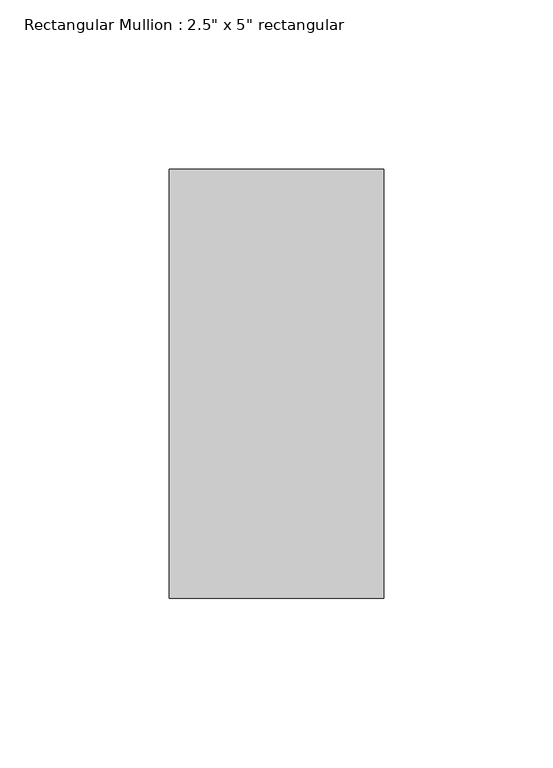
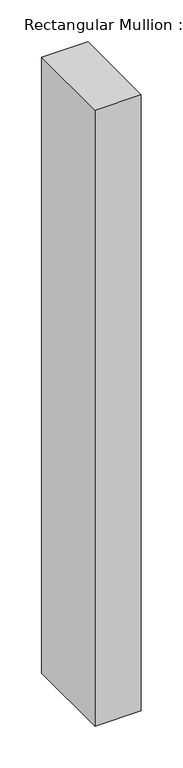
"""IFC4 building model written with IfcOpenShell, lengths in millimetres: member geometry."""

from ifc_helpers import new_model, si_unit, frame, origin, place, context, project, spatial, polyline, outline, extrude, source, transform, mapped, element, save


def member_f1f71bde(model_context):
    return source(origin(), model_context, "Body", "SweptSolid", [
        extrude(outline(polyline([(0.0, 63.5), (0.0, -63.5), (-63.5, -63.5), (-63.5, 63.5), (0.0, 63.5)])), frame((0.0, 0.0, -895.35), z_axis=(0.0, 0.0, 1.0), x_axis=(1.0, 0.0, 0.0)), (0.0, 0.0, 1.0), 895.35),
    ])


if __name__ == "__main__":
    model = new_model("IFC4")
    model_context = context("Model", 3, world=origin())
    ifc_project = project(units=[si_unit("LENGTHUNIT", "METRE", prefix="MILLI")], contexts=[model_context])
    site = spatial("IfcSite", under=ifc_project)
    building = spatial("IfcBuilding", under=site)
    placement = place(None, origin())
    member_shape = member_f1f71bde(model_context)
    element("IfcMember", 1, ObjectType="Rectangular Mullion : 2.5\" x 5\" rectangular", at=placement, inside=building, context=model_context, shape_type="MappedRepresentation", body=[
        mapped(member_shape, transform((0.0, 0.0, 0.0), x_axis=(1.0, 0.0, 0.0), y_axis=(0.0, 1.0, 0.0), z_axis=(0.0, 0.0, 1.0))),
    ])
    save(model, "model.ifc")

# Revit data of these elements
# Type "Rectangular Mullion : 2.5\" x 5\" rectangular"
#   built-in parameter 1007304 = 0.416667 (stored number, unit not read)
#   built-in parameter 1007301 = 0.104167 (stored number, unit not read)
#   built-in parameter 1007300 = 0.104167 (stored number, unit not read)
